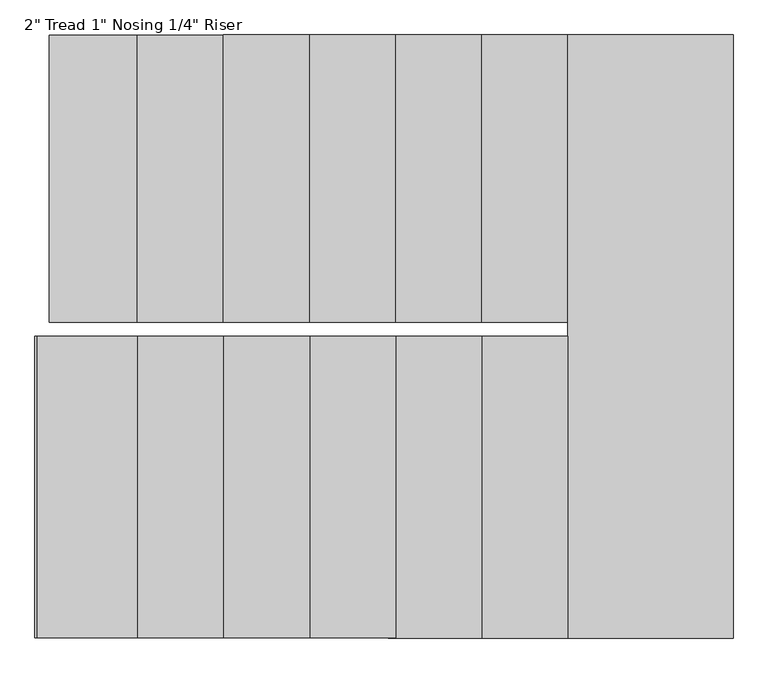
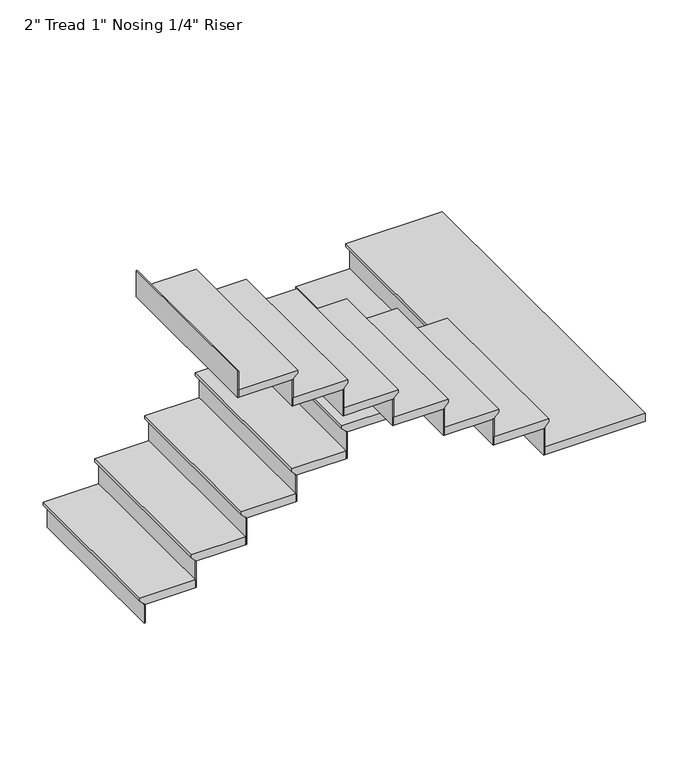
"""IFC4 building model written with IfcOpenShell, lengths in millimetres: stair flight geometry."""

from ifc_helpers import new_model, si_unit, origin, place, context, project, spatial, faceted_brep, source, transform, mapped, element, save


def stair_flight_656f6d92(model_context):
    return source(origin(), model_context, "Body", "Brep", [
        faceted_brep([(-1167.6638307, -167.7482799, 3350.6833333), (-1167.6638307, -167.7482799, 3369.7333333), (-1167.6638307, 848.2517201, 3369.7333333), (-1167.6638307, 848.2517201, 3350.6833333), (-1142.2638307, -167.7482799, 3325.2833333), (-1142.2638307, 848.2517201, 3325.2833333), (-831.1138307, -167.7482799, 3369.7333333), (-831.1138307, 848.2517201, 3369.7333333), (-1142.2638307, 848.2517201, 3318.9333333), (-831.1138307, 848.2517201, 3318.9333333), (-831.1138307, -167.7482799, 3318.9333333), (-1142.2638307, -167.7482799, 3318.9333333)], [[[0, 1, 2, 3]], [[4, 0, 3, 5]], [[2, 1, 6, 7]], [[8, 9, 10, 11]], [[2, 7, 9, 8, 5, 3]], [[8, 11, 4, 5]], [[6, 1, 0, 4, 11, 10]], [[7, 6, 10, 9]]]),
        faceted_brep([(-1142.2638307, -167.7482799, 3318.9333333), (-1142.2638307, -167.7482799, 3200.4), (-1135.9138307, -167.7482799, 3200.4), (-1135.9138307, -167.7482799, 3318.9333333), (-1142.2638307, 848.2517201, 3318.9333333), (-1135.9138307, 848.2517201, 3318.9333333), (-1135.9138307, 848.2517201, 3200.4), (-1142.2638307, 848.2517201, 3200.4)], [[[0, 1, 2, 3]], [[4, 5, 6, 7]], [[1, 0, 4, 7]], [[2, 1, 7, 6]], [[3, 2, 6, 5]], [[0, 3, 5, 4]]]),
        faceted_brep([(-831.1138307, -167.7482799, 3488.2666667), (-831.1138307, -167.7482799, 3318.9333333), (-824.7638307, -167.7482799, 3318.9333333), (-824.7638307, -167.7482799, 3488.2666667), (-831.1138307, 848.2517201, 3488.2666667), (-824.7638307, 848.2517201, 3488.2666667), (-824.7638307, 848.2517201, 3318.9333333), (-831.1138307, 848.2517201, 3318.9333333)], [[[0, 1, 2, 3]], [[4, 5, 6, 7]], [[1, 0, 4, 7]], [[2, 1, 7, 6]], [[3, 2, 6, 5]], [[0, 3, 5, 4]]]),
        faceted_brep([(-856.5138307, 848.2517201, 3539.0666667), (-856.5138307, -167.7482799, 3539.0666667), (-526.3138307, -167.7482799, 3539.0666667), (-526.3138307, 848.2517201, 3539.0666667), (-831.1138307, 848.2517201, 3488.2666667), (-526.3138307, 848.2517201, 3488.2666667), (-526.3138307, -167.7482799, 3488.2666667), (-831.1138307, -167.7482799, 3488.2666667), (-831.1138307, 848.2517201, 3494.6166667), (-856.5138307, 848.2517201, 3520.0166667), (-831.1138307, -167.7482799, 3494.6166667), (-856.5138307, -167.7482799, 3520.0166667)], [[[0, 1, 2, 3]], [[4, 5, 6, 7]], [[0, 3, 5, 4, 8, 9]], [[4, 7, 10, 8]], [[2, 1, 11, 10, 7, 6]], [[3, 2, 6, 5]], [[11, 1, 0, 9]], [[10, 11, 9, 8]]]),
        faceted_brep([(-526.3138307, -167.7482799, 3657.6), (-526.3138307, -167.7482799, 3488.2666667), (-519.9638307, -167.7482799, 3488.2666667), (-519.9638307, -167.7482799, 3657.6), (-526.3138307, 848.2517201, 3657.6), (-519.9638307, 848.2517201, 3657.6), (-519.9638307, 848.2517201, 3488.2666667), (-526.3138307, 848.2517201, 3488.2666667)], [[[0, 1, 2, 3]], [[4, 5, 6, 7]], [[1, 0, 4, 7]], [[2, 1, 7, 6]], [[3, 2, 6, 5]], [[0, 3, 5, 4]]]),
        faceted_brep([(-551.7138307, 848.2517201, 3708.4), (-551.7138307, -167.7482799, 3708.4), (-221.5138307, -167.7482799, 3708.4), (-221.5138307, 848.2517201, 3708.4), (-526.3138307, 848.2517201, 3657.6), (-221.5138307, 848.2517201, 3657.6), (-221.5138307, -167.7482799, 3657.6), (-526.3138307, -167.7482799, 3657.6), (-526.3138307, 848.2517201, 3663.95), (-551.7138307, 848.2517201, 3689.35), (-526.3138307, -167.7482799, 3663.95), (-551.7138307, -167.7482799, 3689.35)], [[[0, 1, 2, 3]], [[4, 5, 6, 7]], [[0, 3, 5, 4, 8, 9]], [[4, 7, 10, 8]], [[2, 1, 11, 10, 7, 6]], [[3, 2, 6, 5]], [[11, 1, 0, 9]], [[10, 11, 9, 8]]]),
        faceted_brep([(-221.5138307, -167.7482799, 3826.9333333), (-221.5138307, -167.7482799, 3657.6), (-215.1638307, -167.7482799, 3657.6), (-215.1638307, -167.7482799, 3826.9333333), (-221.5138307, 848.2517201, 3826.9333333), (-215.1638307, 848.2517201, 3826.9333333), (-215.1638307, 848.2517201, 3657.6), (-221.5138307, 848.2517201, 3657.6)], [[[0, 1, 2, 3]], [[4, 5, 6, 7]], [[1, 0, 4, 7]], [[2, 1, 7, 6]], [[3, 2, 6, 5]], [[0, 3, 5, 4]]]),
        faceted_brep([(-246.9138307, 848.2517201, 3877.7333333), (-246.9138307, -167.7482799, 3877.7333333), (83.2861693, -167.7482799, 3877.7333333), (83.2861693, 848.2517201, 3877.7333333), (-221.5138307, 848.2517201, 3826.9333333), (83.2861693, 848.2517201, 3826.9333333), (83.2861693, -167.7482799, 3826.9333333), (-221.5138307, -167.7482799, 3826.9333333), (-221.5138307, 848.2517201, 3833.2833333), (-246.9138307, 848.2517201, 3858.6833333), (-221.5138307, -167.7482799, 3833.2833333), (-246.9138307, -167.7482799, 3858.6833333)], [[[0, 1, 2, 3]], [[4, 5, 6, 7]], [[0, 3, 5, 4, 8, 9]], [[4, 7, 10, 8]], [[2, 1, 11, 10, 7, 6]], [[3, 2, 6, 5]], [[11, 1, 0, 9]], [[10, 11, 9, 8]]]),
        faceted_brep([(83.2861693, -167.7482799, 3996.2666667), (83.2861693, -167.7482799, 3826.9333333), (89.6361693, -167.7482799, 3826.9333333), (89.6361693, -167.7482799, 3996.2666667), (83.2861693, 848.2517201, 3996.2666667), (89.6361693, 848.2517201, 3996.2666667), (89.6361693, 848.2517201, 3826.9333333), (83.2861693, 848.2517201, 3826.9333333)], [[[0, 1, 2, 3]], [[4, 5, 6, 7]], [[1, 0, 4, 7]], [[2, 1, 7, 6]], [[3, 2, 6, 5]], [[0, 3, 5, 4]]]),
        faceted_brep([(57.8861693, 848.2517201, 4047.0666667), (57.8861693, -167.7482799, 4047.0666667), (388.0861693, -167.7482799, 4047.0666667), (388.0861693, 848.2517201, 4047.0666667), (83.2861693, 848.2517201, 3996.2666667), (388.0861693, 848.2517201, 3996.2666667), (388.0861693, -167.7482799, 3996.2666667), (83.2861693, -167.7482799, 3996.2666667), (83.2861693, 848.2517201, 4002.6166667), (57.8861693, 848.2517201, 4028.0166667), (83.2861693, -167.7482799, 4002.6166667), (57.8861693, -167.7482799, 4028.0166667)], [[[0, 1, 2, 3]], [[4, 5, 6, 7]], [[0, 3, 5, 4, 8, 9]], [[4, 7, 10, 8]], [[2, 1, 11, 10, 7, 6]], [[3, 2, 6, 5]], [[11, 1, 0, 9]], [[10, 11, 9, 8]]]),
        faceted_brep([(388.0861693, -167.7482799, 4165.6), (388.0861693, -167.7482799, 3996.2666667), (394.4361693, -167.7482799, 3996.2666667), (394.4361693, -167.7482799, 4165.6), (388.0861693, 848.2517201, 4165.6), (394.4361693, 848.2517201, 4165.6), (394.4361693, 848.2517201, 3996.2666667), (388.0861693, 848.2517201, 3996.2666667)], [[[0, 1, 2, 3]], [[4, 5, 6, 7]], [[1, 0, 4, 7]], [[2, 1, 7, 6]], [[3, 2, 6, 5]], [[0, 3, 5, 4]]]),
        faceted_brep([(362.6861693, 848.2517201, 4216.4), (362.6861693, -167.7482799, 4216.4), (692.8861693, -167.7482799, 4216.4), (692.8861693, 848.2517201, 4216.4), (388.0861693, 848.2517201, 4165.6), (692.8861693, 848.2517201, 4165.6), (692.8861693, -167.7482799, 4165.6), (388.0861693, -167.7482799, 4165.6), (388.0861693, 848.2517201, 4171.95), (362.6861693, 848.2517201, 4197.35), (388.0861693, -167.7482799, 4171.95), (362.6861693, -167.7482799, 4197.35)], [[[0, 1, 2, 3]], [[4, 5, 6, 7]], [[0, 3, 5, 4, 8, 9]], [[4, 7, 10, 8]], [[2, 1, 11, 10, 7, 6]], [[3, 2, 6, 5]], [[11, 1, 0, 9]], [[10, 11, 9, 8]]]),
        faceted_brep([(692.8861693, -167.7482799, 4334.9333333), (692.8861693, -167.7482799, 4165.6), (699.2361693, -167.7482799, 4165.6), (699.2361693, -167.7482799, 4334.9333333), (692.8861693, 848.2517201, 4334.9333333), (699.2361693, 848.2517201, 4334.9333333), (699.2361693, 848.2517201, 4165.6), (692.8861693, 848.2517201, 4165.6)], [[[0, 1, 2, 3]], [[4, 5, 6, 7]], [[1, 0, 4, 7]], [[2, 1, 7, 6]], [[3, 2, 6, 5]], [[0, 3, 5, 4]]]),
        faceted_brep([(642.0861693, -1285.3482799, 4385.7333333), (1251.6861693, -1285.3482799, 4385.7333333), (1251.6861693, 848.2517201, 4385.7333333), (667.4861693, 848.2517201, 4385.7333333), (667.4861693, -218.5482799, 4385.7333333), (642.0861693, -218.5482799, 4385.7333333), (1251.6861693, -1285.3482799, 4334.9333333), (642.0861693, -1285.3482799, 4334.9333333), (642.0861693, -218.5482799, 4334.9333333), (667.4861693, -218.5482799, 4334.9333333), (667.4861693, -167.7482799, 4334.9333333), (692.8861693, -167.7482799, 4334.9333333), (692.8861693, 848.2517201, 4334.9333333), (1251.6861693, 848.2517201, 4334.9333333), (692.8861693, 848.2517201, 4341.2833333), (667.4861693, 848.2517201, 4366.6833333), (692.8861693, -167.7482799, 4341.2833333), (667.4861693, -167.7482799, 4366.6833333)], [[[0, 1, 2, 3, 4, 5]], [[6, 7, 8, 9, 10, 11, 12, 13]], [[1, 0, 7, 6]], [[2, 1, 6, 13]], [[3, 2, 13, 12, 14, 15]], [[12, 11, 16, 14]], [[11, 10, 17, 16]], [[4, 3, 15, 17, 10, 9]], [[5, 4, 9, 8]], [[0, 5, 8, 7]], [[15, 14, 16, 17]]]),
        faceted_brep([(642.0861693, -218.5482799, 4504.2666667), (642.0861693, -218.5482799, 4334.9333333), (635.7361693, -218.5482799, 4334.9333333), (635.7361693, -218.5482799, 4504.2666667), (642.0861693, -1285.3482799, 4504.2666667), (635.7361693, -1285.3482799, 4504.2666667), (635.7361693, -1285.3482799, 4334.9333333), (642.0861693, -1285.3482799, 4334.9333333)], [[[0, 1, 2, 3]], [[4, 5, 6, 7]], [[1, 0, 4, 7]], [[2, 1, 7, 6]], [[3, 2, 6, 5]], [[0, 3, 5, 4]]]),
        faceted_brep([(667.4861693, -1285.3482799, 4555.0666667), (667.4861693, -218.5482799, 4555.0666667), (337.2861693, -218.5482799, 4555.0666667), (337.2861693, -1285.3482799, 4555.0666667), (642.0861693, -1285.3482799, 4504.2666667), (337.2861693, -1285.3482799, 4504.2666667), (337.2861693, -218.5482799, 4504.2666667), (642.0861693, -218.5482799, 4504.2666667), (642.0861693, -1285.3482799, 4510.6166667), (667.4861693, -1285.3482799, 4536.0166667), (642.0861693, -218.5482799, 4510.6166667), (667.4861693, -218.5482799, 4536.0166667)], [[[0, 1, 2, 3]], [[4, 5, 6, 7]], [[0, 3, 5, 4, 8, 9]], [[4, 7, 10, 8]], [[2, 1, 11, 10, 7, 6]], [[3, 2, 6, 5]], [[11, 1, 0, 9]], [[10, 11, 9, 8]]]),
        faceted_brep([(337.2861693, -218.5482799, 4673.6), (337.2861693, -218.5482799, 4504.2666667), (330.9361693, -218.5482799, 4504.2666667), (330.9361693, -218.5482799, 4673.6), (337.2861693, -1285.3482799, 4673.6), (330.9361693, -1285.3482799, 4673.6), (330.9361693, -1285.3482799, 4504.2666667), (337.2861693, -1285.3482799, 4504.2666667)], [[[0, 1, 2, 3]], [[4, 5, 6, 7]], [[1, 0, 4, 7]], [[2, 1, 7, 6]], [[3, 2, 6, 5]], [[0, 3, 5, 4]]]),
        faceted_brep([(362.6861693, -1285.3482799, 4724.4), (362.6861693, -218.5482799, 4724.4), (32.4861693, -218.5482799, 4724.4), (32.4861693, -1285.3482799, 4724.4), (337.2861693, -1285.3482799, 4673.6), (32.4861693, -1285.3482799, 4673.6), (32.4861693, -218.5482799, 4673.6), (337.2861693, -218.5482799, 4673.6), (337.2861693, -1285.3482799, 4679.95), (362.6861693, -1285.3482799, 4705.35), (337.2861693, -218.5482799, 4679.95), (362.6861693, -218.5482799, 4705.35)], [[[0, 1, 2, 3]], [[4, 5, 6, 7]], [[0, 3, 5, 4, 8, 9]], [[4, 7, 10, 8]], [[2, 1, 11, 10, 7, 6]], [[3, 2, 6, 5]], [[11, 1, 0, 9]], [[10, 11, 9, 8]]]),
        faceted_brep([(32.4861693, -218.5482799, 4842.9333333), (32.4861693, -218.5482799, 4673.6), (26.1361693, -218.5482799, 4673.6), (26.1361693, -218.5482799, 4842.9333333), (32.4861693, -1285.3482799, 4842.9333333), (26.1361693, -1285.3482799, 4842.9333333), (26.1361693, -1285.3482799, 4673.6), (32.4861693, -1285.3482799, 4673.6)], [[[0, 1, 2, 3]], [[4, 5, 6, 7]], [[1, 0, 4, 7]], [[2, 1, 7, 6]], [[3, 2, 6, 5]], [[0, 3, 5, 4]]]),
        faceted_brep([(57.8861693, -1285.3482799, 4893.7333333), (57.8861693, -218.5482799, 4893.7333333), (-272.3138307, -218.5482799, 4893.7333333), (-272.3138307, -1285.3482799, 4893.7333333), (32.4861693, -1285.3482799, 4842.9333333), (-272.3138307, -1285.3482799, 4842.9333333), (-272.3138307, -218.5482799, 4842.9333333), (32.4861693, -218.5482799, 4842.9333333), (32.4861693, -1285.3482799, 4849.2833333), (57.8861693, -1285.3482799, 4874.6833333), (32.4861693, -218.5482799, 4849.2833333), (57.8861693, -218.5482799, 4874.6833333)], [[[0, 1, 2, 3]], [[4, 5, 6, 7]], [[0, 3, 5, 4, 8, 9]], [[4, 7, 10, 8]], [[2, 1, 11, 10, 7, 6]], [[3, 2, 6, 5]], [[11, 1, 0, 9]], [[10, 11, 9, 8]]]),
        faceted_brep([(-272.3138307, -218.5482799, 5012.2666667), (-272.3138307, -218.5482799, 4842.9333333), (-278.6638307, -218.5482799, 4842.9333333), (-278.6638307, -218.5482799, 5012.2666667), (-272.3138307, -1285.3482799, 5012.2666667), (-278.6638307, -1285.3482799, 5012.2666667), (-278.6638307, -1285.3482799, 4842.9333333), (-272.3138307, -1285.3482799, 4842.9333333)], [[[0, 1, 2, 3]], [[4, 5, 6, 7]], [[1, 0, 4, 7]], [[2, 1, 7, 6]], [[3, 2, 6, 5]], [[0, 3, 5, 4]]]),
        faceted_brep([(-246.9138307, -1285.3482799, 5063.0666667), (-246.9138307, -218.5482799, 5063.0666667), (-577.1138307, -218.5482799, 5063.0666667), (-577.1138307, -1285.3482799, 5063.0666667), (-272.3138307, -1285.3482799, 5012.2666667), (-577.1138307, -1285.3482799, 5012.2666667), (-577.1138307, -218.5482799, 5012.2666667), (-272.3138307, -218.5482799, 5012.2666667), (-272.3138307, -1285.3482799, 5018.6166667), (-246.9138307, -1285.3482799, 5044.0166667), (-272.3138307, -218.5482799, 5018.6166667), (-246.9138307, -218.5482799, 5044.0166667)], [[[0, 1, 2, 3]], [[4, 5, 6, 7]], [[0, 3, 5, 4, 8, 9]], [[4, 7, 10, 8]], [[2, 1, 11, 10, 7, 6]], [[3, 2, 6, 5]], [[11, 1, 0, 9]], [[10, 11, 9, 8]]]),
        faceted_brep([(-577.1138307, -218.5482799, 5181.6), (-577.1138307, -218.5482799, 5012.2666667), (-583.4638307, -218.5482799, 5012.2666667), (-583.4638307, -218.5482799, 5181.6), (-577.1138307, -1285.3482799, 5181.6), (-583.4638307, -1285.3482799, 5181.6), (-583.4638307, -1285.3482799, 5012.2666667), (-577.1138307, -1285.3482799, 5012.2666667)], [[[0, 1, 2, 3]], [[4, 5, 6, 7]], [[1, 0, 4, 7]], [[2, 1, 7, 6]], [[3, 2, 6, 5]], [[0, 3, 5, 4]]]),
        faceted_brep([(-551.7138307, -1285.3482799, 5232.4), (-551.7138307, -218.5482799, 5232.4), (-881.9138307, -218.5482799, 5232.4), (-881.9138307, -1285.3482799, 5232.4), (-577.1138307, -1285.3482799, 5181.6), (-881.9138307, -1285.3482799, 5181.6), (-881.9138307, -218.5482799, 5181.6), (-577.1138307, -218.5482799, 5181.6), (-577.1138307, -1285.3482799, 5187.95), (-551.7138307, -1285.3482799, 5213.35), (-577.1138307, -218.5482799, 5187.95), (-551.7138307, -218.5482799, 5213.35)], [[[0, 1, 2, 3]], [[4, 5, 6, 7]], [[0, 3, 5, 4, 8, 9]], [[4, 7, 10, 8]], [[2, 1, 11, 10, 7, 6]], [[3, 2, 6, 5]], [[11, 1, 0, 9]], [[10, 11, 9, 8]]]),
        faceted_brep([(-881.9138307, -218.5482799, 5350.9333333), (-881.9138307, -218.5482799, 5181.6), (-888.2638307, -218.5482799, 5181.6), (-888.2638307, -218.5482799, 5350.9333333), (-881.9138307, -1285.3482799, 5350.9333333), (-888.2638307, -1285.3482799, 5350.9333333), (-888.2638307, -1285.3482799, 5181.6), (-881.9138307, -1285.3482799, 5181.6)], [[[0, 1, 2, 3]], [[4, 5, 6, 7]], [[1, 0, 4, 7]], [[2, 1, 7, 6]], [[3, 2, 6, 5]], [[0, 3, 5, 4]]]),
        faceted_brep([(-1212.1138307, -218.5482799, 5520.2666667), (-1212.1138307, -218.5482799, 5350.9333333), (-1218.4638307, -218.5482799, 5350.9333333), (-1218.4638307, -218.5482799, 5520.2666667), (-1212.1138307, -1285.3482799, 5520.2666667), (-1218.4638307, -1285.3482799, 5520.2666667), (-1218.4638307, -1285.3482799, 5350.9333333), (-1212.1138307, -1285.3482799, 5350.9333333)], [[[0, 1, 2, 3]], [[4, 5, 6, 7]], [[1, 0, 4, 7]], [[2, 1, 7, 6]], [[3, 2, 6, 5]], [[0, 3, 5, 4]]]),
        faceted_brep([(-856.5138307, -1285.3482799, 5401.7333333), (-856.5138307, -218.5482799, 5401.7333333), (-1212.1138307, -218.5482799, 5401.7333333), (-1212.1138307, -1285.3482799, 5401.7333333), (-881.9138307, -1285.3482799, 5350.9333333), (-1212.1138307, -1285.3482799, 5350.9333333), (-1212.1138307, -218.5482799, 5350.9333333), (-881.9138307, -218.5482799, 5350.9333333), (-881.9138307, -1285.3482799, 5357.2833333), (-856.5138307, -1285.3482799, 5382.6833333), (-881.9138307, -218.5482799, 5357.2833333), (-856.5138307, -218.5482799, 5382.6833333)], [[[0, 1, 2, 3]], [[4, 5, 6, 7]], [[0, 3, 5, 4, 8, 9]], [[4, 7, 10, 8]], [[2, 1, 11, 10, 7, 6]], [[3, 2, 6, 5]], [[11, 1, 0, 9]], [[10, 11, 9, 8]]]),
    ])


if __name__ == "__main__":
    model = new_model("IFC4")
    model_context = context("Model", 3, world=origin())
    ifc_project = project(units=[si_unit("LENGTHUNIT", "METRE", prefix="MILLI")], contexts=[model_context])
    site = spatial("IfcSite", under=ifc_project)
    building = spatial("IfcBuilding", under=site)
    placement = place(None, origin())
    stair_flight_shape = stair_flight_656f6d92(model_context)
    element("IfcStairFlight", 1, ObjectType="2\" Tread 1\" Nosing 1/4\" Riser", at=placement, inside=building, context=model_context, shape_type="MappedRepresentation", body=[
        mapped(stair_flight_shape, transform((0.0, 0.0, 0.0), x_axis=(1.0, 0.0, 0.0), y_axis=(0.0, 1.0, 0.0), z_axis=(0.0, 0.0, 1.0))),
    ])
    save(model, "model.ifc")
